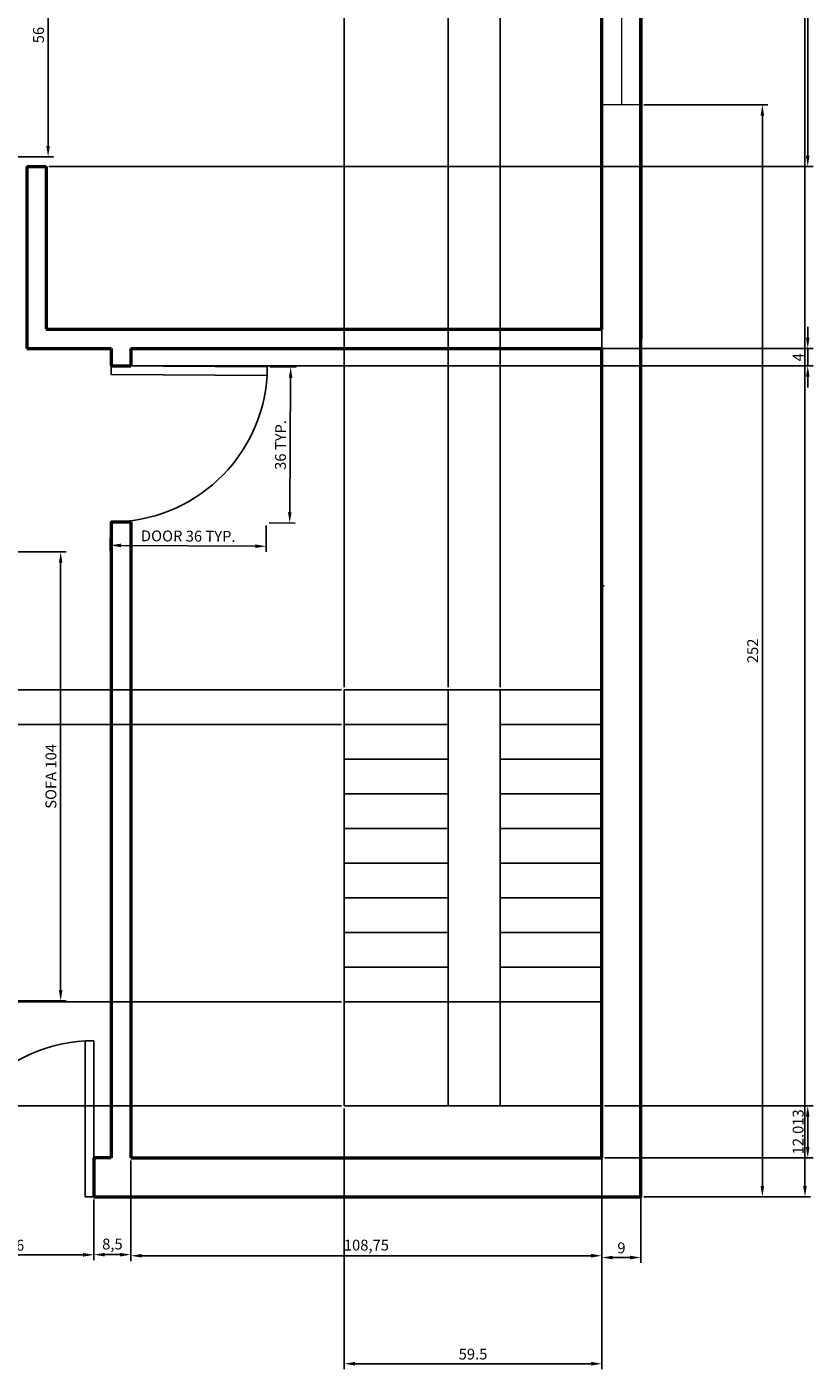
# Model space of a CAD drawing. Units: inches. Extents: x 907 to 2409, y 377 to 1163.
# Tile 3 of 9: x 1197 to 1378, y 377 to 687. Entities that reach past the tile are written whole.
import ezdxf

# ---------------------------------------------------------------- set-up
doc = ezdxf.new("R2010")
doc.units = ezdxf.units.IN
for name, color, linetype, lineweight in [('A-ANNO-DIMS', 2, 'Continuous', 18), ('A-DOOR', 3, 'Continuous', 25), ('A-FLOR-STRS', 7, 'Continuous', 25), ('A-GLAZ', 4, 'Continuous', 18), ('A-WALL', 7, 'Continuous', 50)]:
    doc.layers.add(name, color=color, linetype=linetype, lineweight=lineweight)
doc.styles.get("Standard").update_dxf_attribs({"font": 'arial.ttf'})
doc.dimstyles.new('ISO-25', dxfattribs={"dimtxt": 2.5, "dimasz": 2.5, "dimexe": 1.25, "dimexo": 0.625, "dimtad": 1, "dimtxsty": 'Standard', "dimcen": 2.5, "dimadec": 0, "dimazin": 0, "dimtfac": 1, "dimtmove": 0, "dimatfit": 3, "dimfxl": 1, "dimarcsym": 0})

# ---------------------------------------------------------------- blocks, each defined once
blk = doc.blocks.new('*D19')
at = {"layer": 'A-ANNO-DIMS', "color": 0, "lineweight": -2, "transparency": 16777216}
for p, q in [((1339.24, 668.87), (1367.89, 668.87)), ((1366.64, 666.37), (1366.64, 419.37)), ((1339.24, 416.87), (1367.89, 416.87))]:
    blk.add_line(p, q, dxfattribs=at)
at = {"layer": 'A-ANNO-DIMS', "color": 0, "transparency": 16777216}
for points in [[(1366.22, 666.37), (1367.05, 666.37), (1366.64, 668.87)], [(1366.22, 419.37), (1367.05, 419.37), (1366.64, 416.87)]]:
    blk.add_solid(points, dxfattribs=at)
at = {"layer": 'Defpoints', "color": 0, "transparency": 16777216}
for p in [(1338.61, 668.87), (1338.61, 416.87), (1366.64, 416.87)]:
    blk.add_point(p, dxfattribs=at)
at = {"layer": 'A-ANNO-DIMS', "color": 0, "transparency": 16777216, "insert": (1364.73, 542.87), "char_height": 2.5, "attachment_point": 5, "rotation": 90}
blk.add_mtext('252', dxfattribs=at)
blk = doc.blocks.new('*D20')
at = {"layer": 'A-ANNO-DIMS', "color": 0, "lineweight": -2, "transparency": 16777216}
for p, q in [((1339.24, 1016.87), (1377.72, 1016.87)), ((1376.47, 419.37), (1376.47, 1014.37)), ((1339.24, 416.87), (1377.72, 416.87))]:
    blk.add_line(p, q, dxfattribs=at)
at = {"layer": 'A-ANNO-DIMS', "color": 0, "transparency": 16777216}
for points in [[(1376.05, 1014.37), (1376.88, 1014.37), (1376.47, 1016.87)], [(1376.05, 419.37), (1376.88, 419.37), (1376.47, 416.87)]]:
    blk.add_solid(points, dxfattribs=at)
at = {"layer": 'Defpoints', "color": 0, "transparency": 16777216}
for p in [(1338.61, 1016.87), (1376.47, 1016.87), (1338.61, 416.87)]:
    blk.add_point(p, dxfattribs=at)
at = {"layer": 'A-ANNO-DIMS', "color": 0, "transparency": 16777216, "insert": (1374.56, 716.87), "char_height": 2.5, "attachment_point": 5, "rotation": 90}
blk.add_mtext('600', dxfattribs=at)
blk = doc.blocks.new('*D21')
at = {"layer": 'A-ANNO-DIMS', "color": 0, "lineweight": -2, "transparency": 16777216}
for p, q in [((1329.61, 425.25), (1329.61, 401.63)), ((1338.61, 425.25), (1338.61, 401.63)), ((1332.11, 402.88), (1336.11, 402.88))]:
    blk.add_line(p, q, dxfattribs=at)
at = {"layer": 'A-ANNO-DIMS', "color": 0, "transparency": 16777216}
for points in [[(1332.11, 403.29), (1332.11, 402.46), (1329.61, 402.88)], [(1336.11, 403.29), (1336.11, 402.46), (1338.61, 402.88)]]:
    blk.add_solid(points, dxfattribs=at)
at = {"layer": 'Defpoints', "color": 0, "transparency": 16777216}
for p in [(1329.61, 425.87), (1338.61, 425.87), (1338.61, 402.88)]:
    blk.add_point(p, dxfattribs=at)
at = {"layer": 'A-ANNO-DIMS', "color": 0, "transparency": 16777216, "insert": (1334.11, 404.78), "char_height": 2.5, "attachment_point": 5}
blk.add_mtext('9', dxfattribs=at)
blk = doc.blocks.new('*D22')
at = {"layer": 'A-ANNO-DIMS', "color": 0, "lineweight": -2, "transparency": 16777216}
for p, q in [((1220.86, 425.25), (1220.86, 402.04)), ((1329.61, 425.25), (1329.61, 402.04)), ((1223.36, 403.29), (1327.11, 403.29))]:
    blk.add_line(p, q, dxfattribs=at)
at = {"layer": 'A-ANNO-DIMS', "color": 0, "transparency": 16777216}
for points in [[(1223.36, 403.71), (1223.36, 402.88), (1220.86, 403.29)], [(1327.11, 403.71), (1327.11, 402.88), (1329.61, 403.29)]]:
    blk.add_solid(points, dxfattribs=at)
at = {"layer": 'Defpoints', "color": 0, "transparency": 16777216}
for p in [(1220.86, 425.87), (1329.61, 425.87), (1329.61, 403.29)]:
    blk.add_point(p, dxfattribs=at)
at = {"layer": 'A-ANNO-DIMS', "color": 0, "transparency": 16777216, "insert": (1275.24, 405.42), "char_height": 2.5, "attachment_point": 5}
blk.add_mtext('108,75', dxfattribs=at)
blk = doc.blocks.new('*D23')
at = {"layer": 'A-ANNO-DIMS', "color": 0, "lineweight": -2, "transparency": 16777216}
for p, q in [((1212.36, 416.25), (1212.36, 402.29)), ((1220.86, 416.13), (1220.86, 402.29)), ((1218.36, 403.54), (1214.86, 403.54))]:
    blk.add_line(p, q, dxfattribs=at)
at = {"layer": 'A-ANNO-DIMS', "color": 0, "transparency": 16777216}
for points in [[(1214.86, 403.96), (1214.86, 403.12), (1212.36, 403.54)], [(1218.36, 403.96), (1218.36, 403.12), (1220.86, 403.54)]]:
    blk.add_solid(points, dxfattribs=at)
at = {"layer": 'Defpoints', "color": 0, "transparency": 16777216}
for p in [(1212.36, 416.87), (1220.86, 416.76), (1212.36, 403.54)]:
    blk.add_point(p, dxfattribs=at)
at = {"layer": 'A-ANNO-DIMS', "color": 0, "transparency": 16777216, "insert": (1216.61, 405.67), "char_height": 2.5, "attachment_point": 5}
blk.add_mtext('8,5', dxfattribs=at)
blk = doc.blocks.new('*D24')
at = {"layer": 'A-ANNO-DIMS', "color": 0, "lineweight": -2, "transparency": 16777216}
for p, q in [((1176.36, 416.32), (1176.36, 402.25)), ((1212.36, 416.25), (1212.36, 402.25)), ((1209.86, 403.5), (1178.86, 403.5))]:
    blk.add_line(p, q, dxfattribs=at)
at = {"layer": 'A-ANNO-DIMS', "color": 0, "transparency": 16777216}
for points in [[(1178.86, 403.92), (1178.86, 403.09), (1176.36, 403.5)], [(1209.86, 403.92), (1209.86, 403.09), (1212.36, 403.5)]]:
    blk.add_solid(points, dxfattribs=at)
at = {"layer": 'Defpoints', "color": 0, "transparency": 16777216}
for p in [(1176.36, 416.95), (1212.36, 416.87), (1176.36, 403.5)]:
    blk.add_point(p, dxfattribs=at)
at = {"layer": 'A-ANNO-DIMS', "color": 0, "transparency": 16777216, "insert": (1194.36, 405.4), "char_height": 2.5, "attachment_point": 5}
blk.add_mtext('36', dxfattribs=at)
blk = doc.blocks.new('DOOR-36IN')
for p, q in [((36, 36), (36, 0)), ((36, 0), (34, 0)), ((36, 0), (34, 0))]:
    blk.add_line(p, q)
blk.add_lwpolyline([(36, 36), (34, 36), (34, 0), (36, 0)], close=True)
blk.add_arc((36.06, 0), 36.06, 93.2732, 180)
blk = doc.blocks.new('WIN-48IN')
for p, q in [((9, 48), (0, 48)), ((4.5, 48), (4.5, 0)), ((9, 24), (0, 24)), ((9, 0), (0, 0))]:
    blk.add_line(p, q)
blk = doc.blocks.new('*D43')
at = {"layer": 'A-ANNO-DIMS', "color": 0, "lineweight": -2, "transparency": 16777216}
for p, q in [((1216.14, 572), (1216.1, 565.97)), ((1252.14, 571.78), (1252.1, 565.76)), ((1218.61, 567.21), (1249.61, 567.02))]:
    blk.add_line(p, q, dxfattribs=at)
at = {"layer": 'A-ANNO-DIMS', "color": 0, "transparency": 16777216}
for points in [[(1218.61, 567.62), (1218.61, 566.79), (1216.11, 567.22)], [(1249.61, 567.44), (1249.61, 566.61), (1252.11, 567.01)]]:
    blk.add_solid(points, dxfattribs=at)
at = {"layer": 'Defpoints', "color": 0, "transparency": 16777216}
for p in [(1216.14, 572.62), (1252.14, 572.41), (1252.11, 567.01)]:
    blk.add_point(p, dxfattribs=at)
at = {"layer": 'A-ANNO-DIMS', "color": 0, "transparency": 16777216, "insert": (1234.12, 569.03), "char_height": 2.5, "attachment_point": 5, "rotation": 359.6605}
blk.add_mtext('DOOR 36 TYP.', dxfattribs=at)
blk = doc.blocks.new('*D44')
at = {"layer": 'A-ANNO-DIMS', "color": 0, "lineweight": -2, "transparency": 16777216}
for p, q in [((1252.98, 608.4), (1259.01, 608.37)), ((1257.56, 574.88), (1257.74, 605.88)), ((1252.77, 572.4), (1258.79, 572.37))]:
    blk.add_line(p, q, dxfattribs=at)
at = {"layer": 'A-ANNO-DIMS', "color": 0, "transparency": 16777216}
for points in [[(1257.33, 605.88), (1258.16, 605.87), (1257.76, 608.38)], [(1257.14, 574.88), (1257.97, 574.87), (1257.54, 572.38)]]:
    blk.add_solid(points, dxfattribs=at)
at = {"layer": 'Defpoints', "color": 0, "transparency": 16777216}
for p in [(1252.36, 608.41), (1257.76, 608.38), (1252.14, 572.41)]:
    blk.add_point(p, dxfattribs=at)
at = {"layer": 'A-ANNO-DIMS', "color": 0, "transparency": 16777216, "insert": (1255.75, 590.39), "char_height": 2.5, "attachment_point": 5, "rotation": 89.6605}
blk.add_mtext('36 TYP.', dxfattribs=at)
blk = doc.blocks.new('*D55')
at = {"layer": 'A-ANNO-DIMS', "color": 0, "lineweight": -2, "transparency": 16777216}
for p, q in [((1189.76, 565.7), (1205.92, 565.7)), ((1204.67, 563.2), (1204.67, 464.62)), ((1189.76, 462.12), (1205.92, 462.12))]:
    blk.add_line(p, q, dxfattribs=at)
at = {"layer": 'A-ANNO-DIMS', "color": 0, "transparency": 16777216}
for points in [[(1204.25, 563.2), (1205.09, 563.2), (1204.67, 565.7)], [(1204.25, 464.62), (1205.09, 464.62), (1204.67, 462.12)]]:
    blk.add_solid(points, dxfattribs=at)
at = {"layer": 'Defpoints', "color": 0, "transparency": 16777216}
for p in [(1189.13, 565.7), (1189.13, 462.12), (1204.67, 462.12)]:
    blk.add_point(p, dxfattribs=at)
at = {"layer": 'A-ANNO-DIMS', "color": 0, "transparency": 16777216, "insert": (1202.75, 513.91), "char_height": 2.5, "attachment_point": 5, "rotation": 90}
blk.add_mtext('SOFA 104', dxfattribs=at)
blk = doc.blocks.new('*D58')
at = {"layer": 'A-ANNO-DIMS', "color": 0, "lineweight": -2, "transparency": 16777216}
for p, q in [((1191.96, 713.06), (1203.02, 713.06)), ((1201.77, 659.4), (1201.77, 710.56)), ((1191.96, 656.9), (1203.02, 656.9))]:
    blk.add_line(p, q, dxfattribs=at)
at = {"layer": 'A-ANNO-DIMS', "color": 0, "transparency": 16777216}
for points in [[(1201.36, 710.56), (1202.19, 710.56), (1201.77, 713.06)], [(1201.36, 659.4), (1202.19, 659.4), (1201.77, 656.9)]]:
    blk.add_solid(points, dxfattribs=at)
at = {"layer": 'Defpoints', "color": 0, "transparency": 16777216}
for p in [(1191.34, 713.06), (1201.77, 713.06), (1191.34, 656.9)]:
    blk.add_point(p, dxfattribs=at)
at = {"layer": 'A-ANNO-DIMS', "color": 0, "transparency": 16777216, "insert": (1199.87, 684.98), "char_height": 2.5, "attachment_point": 5, "rotation": 90}
blk.add_mtext('56', dxfattribs=at)
blk = doc.blocks.new('*D63')
at = {"layer": 'A-ANNO-DIMS', "color": 0, "lineweight": -2, "transparency": 16777216}
for p, q in [((1270.1, 437.26), (1270.1, 377.12)), ((1329.6, 437.26), (1329.6, 377.12)), ((1272.6, 378.37), (1327.1, 378.37))]:
    blk.add_line(p, q, dxfattribs=at)
at = {"layer": 'A-ANNO-DIMS', "color": 0, "transparency": 16777216}
for points in [[(1272.6, 378.79), (1272.6, 377.95), (1270.1, 378.37)], [(1327.1, 378.79), (1327.1, 377.95), (1329.6, 378.37)]]:
    blk.add_solid(points, dxfattribs=at)
at = {"layer": 'Defpoints', "color": 0, "transparency": 16777216}
for p in [(1270.1, 437.88), (1329.6, 437.88), (1329.6, 378.37)]:
    blk.add_point(p, dxfattribs=at)
at = {"layer": 'A-ANNO-DIMS', "color": 0, "transparency": 16777216, "insert": (1299.85, 380.27), "char_height": 2.5, "attachment_point": 5}
blk.add_mtext('59.5', dxfattribs=at)
blk = doc.blocks.new('*D64')
at = {"layer": 'A-ANNO-DIMS', "color": 0, "lineweight": -2, "transparency": 16777216}
for p, q in [((1269.47, 533.88), (938.33, 533.88)), ((939.58, 440.38), (939.58, 531.38)), ((1269.47, 437.88), (938.33, 437.88))]:
    blk.add_line(p, q, dxfattribs=at)
at = {"layer": 'A-ANNO-DIMS', "color": 0, "transparency": 16777216}
for points in [[(939.17, 531.38), (940, 531.38), (939.58, 533.88)], [(939.17, 440.38), (940, 440.38), (939.58, 437.88)]]:
    blk.add_solid(points, dxfattribs=at)
at = {"layer": 'Defpoints', "color": 0, "transparency": 16777216}
for p in [(939.58, 533.88), (1270.1, 533.88), (1270.1, 437.88)]:
    blk.add_point(p, dxfattribs=at)
at = {"layer": 'A-ANNO-DIMS', "color": 0, "transparency": 16777216, "insert": (937.68, 485.88), "char_height": 2.5, "attachment_point": 5, "rotation": 90}
blk.add_mtext('96', dxfattribs=at)
blk = doc.blocks.new('*D65')
at = {"layer": 'A-ANNO-DIMS', "color": 0, "lineweight": -2, "transparency": 16777216}
for p, q in [((1330.23, 437.88), (1378.36, 437.88)), ((1377.11, 428.37), (1377.11, 435.38)), ((1330.24, 425.87), (1378.36, 425.87))]:
    blk.add_line(p, q, dxfattribs=at)
at = {"layer": 'A-ANNO-DIMS', "color": 0, "transparency": 16777216}
for points in [[(1376.7, 435.38), (1377.53, 435.38), (1377.11, 437.88)], [(1376.7, 428.37), (1377.53, 428.37), (1377.11, 425.87)]]:
    blk.add_solid(points, dxfattribs=at)
at = {"layer": 'Defpoints', "color": 0, "transparency": 16777216}
for p in [(1329.6, 437.88), (1377.11, 437.88), (1329.61, 425.87)]:
    blk.add_point(p, dxfattribs=at)
at = {"layer": 'A-ANNO-DIMS', "color": 0, "transparency": 16777216, "insert": (1375.21, 431.88), "char_height": 2.5, "attachment_point": 5, "rotation": 90}
blk.add_mtext('12.013', dxfattribs=at)
blk = doc.blocks.new('*D74')
at = {"layer": 'A-ANNO-DIMS', "color": 0, "lineweight": -2, "transparency": 16777216}
for p, q in [((1201.97, 726.62), (1378.36, 726.62)), ((1377.11, 657.12), (1377.11, 724.12)), ((1201.97, 654.62), (1378.36, 654.62))]:
    blk.add_line(p, q, dxfattribs=at)
at = {"layer": 'A-ANNO-DIMS', "color": 0, "transparency": 16777216}
for points in [[(1376.7, 724.12), (1377.53, 724.12), (1377.11, 726.62)], [(1376.7, 657.12), (1377.53, 657.12), (1377.11, 654.62)]]:
    blk.add_solid(points, dxfattribs=at)
at = {"layer": 'Defpoints', "color": 0, "transparency": 16777216}
for p in [(1201.34, 726.62), (1377.11, 726.62), (1201.34, 654.62)]:
    blk.add_point(p, dxfattribs=at)
at = {"layer": 'A-ANNO-DIMS', "color": 0, "transparency": 16777216, "insert": (1375.23, 690.62), "char_height": 2.5, "attachment_point": 5, "rotation": 90}
blk.add_mtext('72', dxfattribs=at)
blk = doc.blocks.new('*D76')
at = {"layer": 'A-ANNO-DIMS', "color": 0, "lineweight": -2, "transparency": 16777216}
for p, q in [((1269.47, 533.88), (938.33, 533.88)), ((939.58, 531.38), (939.58, 528.38)), ((1269.47, 525.88), (938.33, 525.88))]:
    blk.add_line(p, q, dxfattribs=at)
at = {"layer": 'A-ANNO-DIMS', "color": 0, "transparency": 16777216}
for points in [[(939.17, 531.38), (940, 531.38), (939.58, 533.88)], [(939.17, 528.38), (940, 528.38), (939.58, 525.88)]]:
    blk.add_solid(points, dxfattribs=at)
at = {"layer": 'Defpoints', "color": 0, "transparency": 16777216}
for p in [(1270.1, 533.88), (939.58, 525.88), (1270.1, 525.88)]:
    blk.add_point(p, dxfattribs=at)
at = {"layer": 'A-ANNO-DIMS', "color": 0, "transparency": 16777216, "insert": (937.68, 529.88), "char_height": 2.5, "attachment_point": 5, "rotation": 90}
blk.add_mtext('8', dxfattribs=at)
blk = doc.blocks.new('*D77')
at = {"layer": 'A-ANNO-DIMS', "color": 0, "lineweight": -2, "transparency": 16777216}
for p, q in [((1270.1, 534.51), (1270.1, 1056.62)), ((1294.1, 534.51), (1294.1, 1056.62)), ((1272.6, 1055.37), (1291.6, 1055.37))]:
    blk.add_line(p, q, dxfattribs=at)
at = {"layer": 'A-ANNO-DIMS', "color": 0, "transparency": 16777216}
for points in [[(1272.6, 1055.79), (1272.6, 1054.95), (1270.1, 1055.37)], [(1291.6, 1055.79), (1291.6, 1054.95), (1294.1, 1055.37)]]:
    blk.add_solid(points, dxfattribs=at)
at = {"layer": 'Defpoints', "color": 0, "transparency": 16777216}
for p in [(1294.1, 1055.37), (1270.1, 533.88), (1294.1, 533.88)]:
    blk.add_point(p, dxfattribs=at)
at = {"layer": 'A-ANNO-DIMS', "color": 0, "transparency": 16777216, "insert": (1282.1, 1057.25), "char_height": 2.5, "attachment_point": 5}
blk.add_mtext('24', dxfattribs=at)
blk = doc.blocks.new('*D78')
at = {"layer": 'A-ANNO-DIMS', "color": 0, "lineweight": -2, "transparency": 16777216}
for p, q in [((1306.1, 534.51), (1306.1, 1056.62)), ((1329.61, 534.51), (1329.61, 1056.62)), ((1308.6, 1055.37), (1327.11, 1055.37))]:
    blk.add_line(p, q, dxfattribs=at)
at = {"layer": 'A-ANNO-DIMS', "color": 0, "transparency": 16777216}
for points in [[(1308.6, 1055.79), (1308.6, 1054.95), (1306.1, 1055.37)], [(1327.11, 1055.79), (1327.11, 1054.95), (1329.61, 1055.37)]]:
    blk.add_solid(points, dxfattribs=at)
at = {"layer": 'Defpoints', "color": 0, "transparency": 16777216}
for p in [(1329.61, 1055.37), (1306.1, 533.88), (1329.61, 533.88)]:
    blk.add_point(p, dxfattribs=at)
at = {"layer": 'A-ANNO-DIMS', "color": 0, "transparency": 16777216, "insert": (1317.86, 1057.27), "char_height": 2.5, "attachment_point": 5}
blk.add_mtext('23.514', dxfattribs=at)
blk = doc.blocks.new('*D79')
at = {"layer": 'A-ANNO-DIMS', "color": 0, "lineweight": -2, "transparency": 16777216}
for p, q in [((1269.47, 461.88), (938.33, 461.88)), ((939.58, 440.38), (939.58, 459.38)), ((1269.47, 437.88), (938.33, 437.88))]:
    blk.add_line(p, q, dxfattribs=at)
at = {"layer": 'A-ANNO-DIMS', "color": 0, "transparency": 16777216}
for points in [[(939.17, 459.38), (940, 459.38), (939.58, 461.88)], [(939.17, 440.38), (940, 440.38), (939.58, 437.88)]]:
    blk.add_solid(points, dxfattribs=at)
at = {"layer": 'Defpoints', "color": 0, "transparency": 16777216}
for p in [(939.58, 461.88), (1270.1, 461.88), (1270.1, 437.88)]:
    blk.add_point(p, dxfattribs=at)
at = {"layer": 'A-ANNO-DIMS', "color": 0, "transparency": 16777216, "insert": (937.7, 449.88), "char_height": 2.5, "attachment_point": 5, "rotation": 90}
blk.add_mtext('24', dxfattribs=at)
blk = doc.blocks.new('*D80')
at = {"layer": 'A-ANNO-DIMS', "color": 0, "lineweight": -2, "transparency": 16777216}
for p, q in [((1377.11, 615.12), (1377.11, 617.62)), ((1221.49, 612.62), (1378.36, 612.62)), ((1377.11, 608.62), (1377.11, 612.62)), ((1221.49, 608.62), (1378.36, 608.62)), ((1377.11, 606.12), (1377.11, 603.62))]:
    blk.add_line(p, q, dxfattribs=at)
at = {"layer": 'A-ANNO-DIMS', "color": 0, "transparency": 16777216}
for points in [[(1376.7, 615.12), (1377.53, 615.12), (1377.11, 612.62)], [(1376.7, 606.12), (1377.53, 606.12), (1377.11, 608.62)]]:
    blk.add_solid(points, dxfattribs=at)
at = {"layer": 'Defpoints', "color": 0, "transparency": 16777216}
for p in [(1220.86, 612.62), (1377.11, 612.62), (1220.86, 608.62)]:
    blk.add_point(p, dxfattribs=at)
at = {"layer": 'A-ANNO-DIMS', "color": 0, "transparency": 16777216, "insert": (1375.24, 610.62), "char_height": 2.5, "attachment_point": 5, "rotation": 90}
blk.add_mtext('4', dxfattribs=at)

msp = doc.modelspace()

# ---------------------------------------------------------------- linework, layer by layer
at = {"layer": 'A-FLOR-STRS'}
for p, q in [((1330.0979, 557.8833), (1329.6122, 557.8833)), ((1270.0979, 533.8833), (1270.0979, 437.8833)), ((1270.0979, 533.8833), (1294.0979, 533.8833)), ((1294.0979, 533.8833), (1294.0979, 437.8833)), ((1294.0979, 533.8833), (1306.0979, 533.8833)), ((1306.0979, 533.8833), (1306.0979, 437.8833)), ((1306.0979, 533.8833), (1329.6122, 533.8833)), ((1270.0979, 525.8833), (1294.0979, 525.8833)), ((1270.0979, 525.8833), (1294.0979, 525.8833)), ((1306.0979, 525.8833), (1329.6122, 525.8833)), ((1306.0979, 525.8833), (1329.6122, 525.8833)), ((1270.0979, 517.8833), (1294.0979, 517.8833)), ((1270.0979, 517.8833), (1294.0979, 517.8833)), ((1306.0979, 517.8833), (1329.6122, 517.8833)), ((1306.0979, 517.8833), (1329.6122, 517.8833)), ((1270.0979, 509.8833), (1294.0979, 509.8833)), ((1270.0979, 509.8833), (1294.0979, 509.8833)), ((1306.0979, 509.8833), (1329.6122, 509.8833)), ((1306.0979, 509.8833), (1329.6122, 509.8833)), ((1270.0979, 501.8833), (1294.0979, 501.8833)), ((1270.0979, 501.8833), (1294.0979, 501.8833)), ((1306.0979, 501.8833), (1329.6122, 501.8833)), ((1306.0979, 501.8833), (1329.6122, 501.8833)), ((1270.0979, 493.8833), (1294.0979, 493.8833)), ((1270.0979, 493.8833), (1294.0979, 493.8833)), ((1306.0979, 493.8833), (1329.6122, 493.8833)), ((1306.0979, 493.8833), (1329.6122, 493.8833)), ((1270.0979, 485.8833), (1294.0979, 485.8833)), ((1270.0979, 485.8833), (1294.0979, 485.8833)), ((1306.0979, 485.8833), (1329.6122, 485.8833)), ((1306.0979, 485.8833), (1329.6122, 485.8833)), ((1270.0979, 477.8833), (1294.0979, 477.8833)), ((1270.0979, 477.8833), (1294.0979, 477.8833)), ((1306.0979, 477.8833), (1329.6122, 477.8833)), ((1306.0979, 477.8833), (1329.6122, 477.8833)), ((1270.0979, 469.8833), (1294.0979, 469.8833)), ((1270.0979, 469.8833), (1294.0979, 469.8833)), ((1306.0979, 469.8833), (1329.6122, 469.8833)), ((1306.0979, 469.8833), (1329.6122, 469.8833)), ((1270.0979, 461.8833), (1329.6029, 461.8833)), ((1270.0979, 461.8833), (1294.0979, 461.8833)), ((1306.0979, 461.8833), (1329.6122, 461.8833)), ((1270.0979, 437.8833), (1329.6029, 437.8833))]:
    msp.add_line(p, q, dxfattribs=at)
at = {"layer": 'A-WALL'}
for p, q in [((1338.6122, 416.8705), (1338.6122, 1016.8705)), ((1338.6122, 416.8705), (1338.6122, 1016.8705)), ((1329.6122, 617.1205), (1329.6122, 768.6205)), ((1338.6122, 770.8705), (1338.6122, 614.8705)), ((1196.8622, 654.6205), (1201.3421, 654.6205)), ((1196.8622, 654.6205), (1196.8622, 612.6205)), ((1201.3421, 654.6205), (1201.3421, 617.1205)), ((1201.3421, 617.1205), (1329.6122, 617.1205)), ((1196.8622, 612.6205), (1216.3622, 612.6205)), ((1216.3622, 612.6205), (1216.3622, 608.6205)), ((1220.8622, 612.6205), (1220.8622, 608.6205)), ((1220.8622, 612.6205), (1329.6122, 612.6205)), ((1329.6122, 425.8705), (1329.6122, 612.6205)), ((1216.3622, 608.6205), (1220.8622, 608.6205)), ((1216.3622, 572.6205), (1220.8622, 572.6205)), ((1216.3622, 572.6205), (1216.3622, 425.8705)), ((1220.8622, 572.6205), (1220.8622, 425.8705)), ((1212.3622, 425.8705), (1212.3622, 416.8705)), ((1216.3622, 425.8705), (1212.3622, 425.8705)), ((1220.8622, 425.8705), (1329.6122, 425.8705)), ((1212.3622, 416.8705), (1216.3622, 416.8705)), ((1216.3622, 416.8705), (1338.6122, 416.8705)), ((1216.3622, 416.8705), (1338.6122, 416.8705))]:
    msp.add_line(p, q, dxfattribs=at)
msp.add_lwpolyline([(1216.3622, 416.8705), (1338.6122, 416.8705), (1338.6122, 1016.8705), (978.6122, 1016.8705), (978.6122, 416.8705), (1100.8622, 416.8705)], dxfattribs=at)

# ---------------------------------------------------------------- block references
at = {"layer": 'A-DOOR', "extrusion": (0, 0, -1), "zscale": -1, "rotation": 90.3395377077909}
msp.add_blockref('DOOR-36IN', (-1216.1441, 572.6212), dxfattribs=at)
at = {"layer": 'A-DOOR'}
msp.add_blockref('DOOR-36IN', (1176.3622, 416.8705), dxfattribs=at)
at = {"layer": 'A-GLAZ'}
msp.add_blockref('WIN-48IN', (1329.612, 668.871), dxfattribs=at)

# ---------------------------------------------------------------- dimensions: what is measured, and where the dimension line sits
at = {"layer": 'A-ANNO-DIMS'}
for base, p1, p2, override, picture, middle in [((1294.0979, 1055.3705), (1270.0979, 533.8833), (1294.0979, 533.8833), {"dimdec": 0, "dimlfac": 1, "dimrnd": 0, "dimzin": 0, "dimdsep": 46, "dimlunit": 2}, '*D77', (1282.0979, 1057.2507)), ((1329.6122, 1055.3705), (1306.0979, 533.8833), (1329.6122, 533.8833), {"dimdec": 3, "dimlfac": 1, "dimrnd": 0, "dimzin": 0, "dimdsep": 46, "dimlunit": 2}, '*D78', (1317.8551, 1057.2728)), ((1329.6029, 378.3705), (1270.0979, 437.8833), (1329.6029, 437.8833), {"dimdec": 1, "dimlfac": 1, "dimrnd": 0, "dimzin": 0, "dimdsep": 46, "dimlunit": 2}, '*D63', (1299.8504, 380.272)), ((1329.6122, 403.293), (1220.8622, 425.8705), (1329.6122, 425.8705), {"dimclrd": 0, "dimclre": 0, "dimclrt": 0}, '*D22', (1275.2372, 405.4203)), ((1338.6122, 402.8763), (1329.6122, 425.8705), (1338.6122, 425.8705), {"dimclrd": 0, "dimclre": 0, "dimclrt": 0}, '*D21', (1334.1122, 404.7777)), ((1176.3622, 403.5018), (1212.3622, 416.8705), (1176.3622, 416.945), {"dimclrd": 0, "dimclre": 0, "dimclrt": 0}, '*D24', (1194.3622, 405.4041)), ((1212.3622, 403.5417), (1220.8622, 416.7578), (1212.3622, 416.8705), {"dimclrd": 0, "dimclre": 0, "dimclrt": 0}, '*D23', (1216.6122, 405.669))]:
    dim = msp.add_linear_dim(base=base, p1=p1, p2=p2, dimstyle='ISO-25', override=override, dxfattribs=at)
    dim.commit()
    dim.dimension.update_dxf_attribs({"geometry": picture, "text_midpoint": middle})
for base, p1, p2, override, picture, middle in [((1376.4651, 1016.8705), (1338.6122, 416.8705), (1338.6122, 1016.8705), {"dimclrd": 0, "dimclre": 0, "dimclrt": 0}, '*D20', (1374.5637, 716.8705)), ((1377.1122, 726.6205), (1201.3421, 654.6205), (1201.3421, 726.6205), {"dimdec": 0, "dimlfac": 1, "dimrnd": 0, "dimzin": 0, "dimdsep": 46, "dimlunit": 2}, '*D74', (1375.2321, 690.6205)), ((1201.775, 713.0624), (1191.3372, 656.8985), (1191.3372, 713.0624), {"dimdec": 0, "dimlfac": 1, "dimrnd": 0, "dimzin": 0, "dimdsep": 46, "dimlunit": 2}, '*D58', (1199.8735, 684.9804)), ((1366.6363, 416.8705), (1338.6122, 668.8705), (1338.6122, 416.8705), {"dimclrd": 0, "dimclre": 0, "dimclrt": 0}, '*D19', (1364.7349, 542.8705)), ((1377.1122, 612.6205), (1220.8622, 608.6205), (1220.8622, 612.6205), {"dimdec": 0, "dimlfac": 1, "dimrnd": 0, "dimzin": 0, "dimdsep": 46, "dimlunit": 2}, '*D80', (1375.2372, 610.6205)), ((939.5829, 533.8833), (1270.0979, 437.8833), (1270.0979, 533.8833), {"dimdec": 0, "dimlfac": 1, "dimrnd": 0, "dimzin": 0, "dimdsep": 46, "dimlunit": 2}, '*D64', (937.6815, 485.8833)), ((939.5829, 525.8833), (1270.0979, 533.8833), (1270.0979, 525.8833), {"dimdec": 0, "dimlfac": 1, "dimrnd": 0, "dimzin": 0, "dimdsep": 46, "dimlunit": 2}, '*D76', (937.6815, 529.8833)), ((939.5829, 461.8833), (1270.0979, 437.8833), (1270.0979, 461.8833), {"dimdec": 0, "dimlfac": 1, "dimrnd": 0, "dimzin": 0, "dimdsep": 46, "dimlunit": 2}, '*D79', (937.7028, 449.8833)), ((1377.1122, 437.8833), (1329.6122, 425.8705), (1329.6029, 437.8833), {"dimdec": 3, "dimlfac": 1, "dimrnd": 0, "dimzin": 0, "dimdsep": 46, "dimlunit": 2}, '*D65', (1375.2099, 431.8769))]:
    dim = msp.add_linear_dim(base=base, p1=p1, p2=p2, angle=90, dimstyle='ISO-25', override=override, dxfattribs=at)
    dim.commit()
    dim.dimension.update_dxf_attribs({"geometry": picture, "text_midpoint": middle})
for base, p1, p2, angle, text, picture, middle in [((1257.7568, 608.3752), (1252.1435, 572.4079), (1252.3568, 608.4072), 89.660462, '<> TYP.', '*D44', (1255.7478, 590.3868)), ((1252.1115, 567.008), (1216.1441, 572.6212), (1252.1435, 572.4079), 359.660462, 'DOOR <> TYP.', '*D43', (1234.1232, 569.0339)), ((1204.6687, 462.12), (1189.131, 565.7049), (1189.131, 462.12), 270, 'SOFA <>', '*D55', (1202.7502, 513.9124))]:
    dim = msp.add_linear_dim(base=base, p1=p1, p2=p2, angle=angle, text=text, dimstyle='ISO-25', override={"dimdec": 0, "dimlfac": 1, "dimrnd": 0, "dimzin": 0, "dimdsep": 46, "dimlunit": 2}, dxfattribs=at)
    dim.commit()
    dim.dimension.update_dxf_attribs({"geometry": picture, "text_midpoint": middle})

doc.saveas('drawing.dxf')
